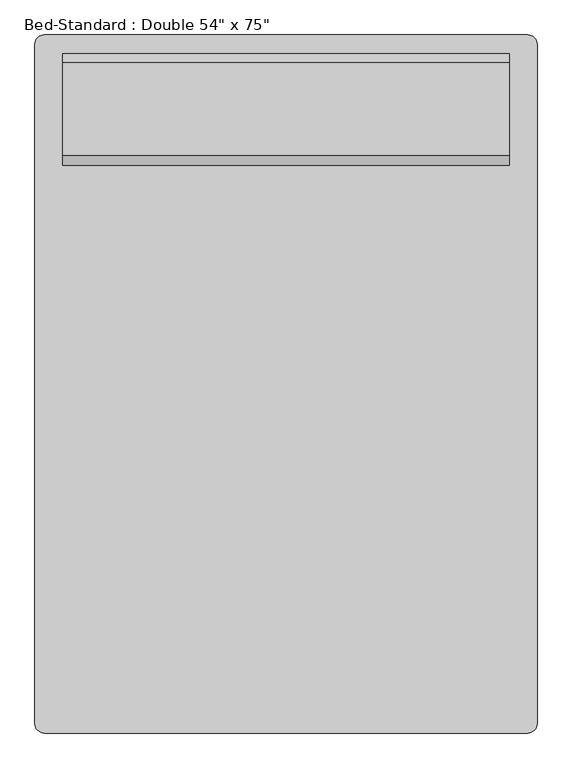
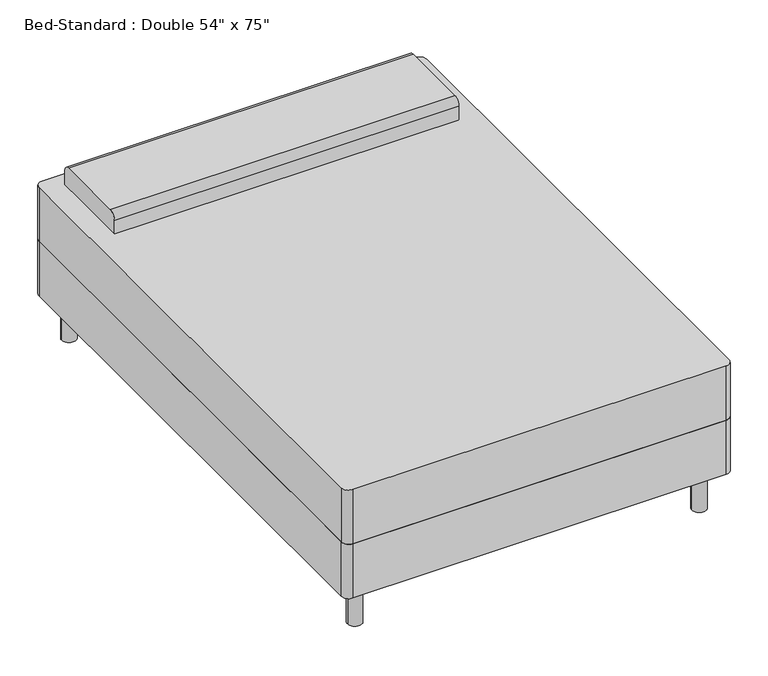
"""IFC4 building model written with IfcOpenShell, lengths in millimetres: furniture geometry."""

from ifc_helpers import new_model, si_unit, point, frame, frame_2d, origin, origin_with_axes, place, context, project, spatial, polyline, circle_curve, trimmed, segment, composite_curve, outline, extrude, source, transform, mapped, element, save


def furniture_0253826f(model_context):
    return source(origin(), model_context, "Body", "SweptSolid", [
        extrude(outline(composite_curve([segment(polyline([(-414.3114754, -972.695082), (-414.3114754, 881.504918)]), True, "CONTINUOUS"), segment(trimmed(circle_curve(frame_2d((-388.9114754, 881.504918)), 25.4), [point((-414.3114754, 881.504918))], [point((-388.9114754, 906.904918))], False, "CARTESIAN"), True, "CONTINUOUS"), segment(polyline([(-388.9114754, 906.904918), (931.8885246, 906.904918)]), True, "CONTINUOUS"), segment(trimmed(circle_curve(frame_2d((931.8885246, 881.504918)), 25.4), [point((931.8885246, 906.904918))], [point((957.2885246, 881.504918))], False, "CARTESIAN"), True, "CONTINUOUS"), segment(polyline([(957.2885246, 881.504918), (957.2885246, -972.695082)]), True, "CONTINUOUS"), segment(trimmed(circle_curve(frame_2d((931.8885246, -972.695082)), 25.4), [point((957.2885246, -972.695082))], [point((931.8885246, -998.095082))], False, "CARTESIAN"), True, "CONTINUOUS"), segment(polyline([(931.8885246, -998.095082), (-388.9114754, -998.095082)]), True, "CONTINUOUS"), segment(trimmed(circle_curve(frame_2d((-388.9114754, -972.695082)), 25.4), [point((-388.9114754, -998.095082))], [point((-414.3114754, -972.695082))], False, "CARTESIAN"), True, "CONTINUOUS")], self_intersect=False)), frame((0.0, 0.0, 152.4), z_axis=(0.0, 0.0, 1.0), x_axis=(1.0, 0.0, 0.0)), (0.0, 0.0, 1.0), 203.2),
        extrude(outline(composite_curve([segment(polyline([(551.304918, 558.8), (551.304918, 609.6)]), True, "CONTINUOUS"), segment(trimmed(circle_curve(frame_2d((576.704918, 609.6)), 25.4), [point((551.304918, 609.6))], [point((576.704918, 635.0))], False, "CARTESIAN"), True, "CONTINUOUS"), segment(polyline([(576.704918, 635.0), (830.704918, 635.0)]), True, "CONTINUOUS"), segment(trimmed(circle_curve(frame_2d((830.704918, 609.6)), 25.4), [point((830.704918, 635.0))], [point((856.104918, 609.6))], False, "CARTESIAN"), True, "CONTINUOUS"), segment(polyline([(856.104918, 609.6), (856.104918, 558.8), (551.304918, 558.8)]), True, "CONTINUOUS")], self_intersect=False)), frame((-338.1114754, 0.0, 0.0), z_axis=(1.0, 0.0, 0.0), x_axis=(0.0, 1.0, 0.0)), (0.0, 0.0, 1.0), 1219.2),
        extrude(outline(composite_curve([segment(trimmed(circle_curve(frame_2d((-338.1114754, 830.704918)), 25.4), [point((-363.5114754, 830.704918))], [point((-312.7114754, 830.704918))], False, "CARTESIAN"), True, "CONTINUOUS"), segment(trimmed(circle_curve(frame_2d((-338.1114754, 830.704918)), 25.4), [point((-312.7114754, 830.704918))], [point((-363.5114754, 830.704918))], False, "CARTESIAN"), True, "CONTINUOUS")], self_intersect=False)), origin_with_axes(), (0.0, 0.0, 1.0), 152.4),
        extrude(outline(composite_curve([segment(trimmed(circle_curve(frame_2d((881.0885246, 830.704918)), 25.4), [point((855.6885246, 830.704918))], [point((906.4885246, 830.704918))], False, "CARTESIAN"), True, "CONTINUOUS"), segment(trimmed(circle_curve(frame_2d((881.0885246, 830.704918)), 25.4), [point((906.4885246, 830.704918))], [point((855.6885246, 830.704918))], False, "CARTESIAN"), True, "CONTINUOUS")], self_intersect=False)), origin_with_axes(), (0.0, 0.0, 1.0), 152.4),
        extrude(outline(composite_curve([segment(trimmed(circle_curve(frame_2d((881.0885246, -921.895082)), 25.4), [point((855.6885246, -921.895082))], [point((906.4885246, -921.895082))], False, "CARTESIAN"), True, "CONTINUOUS"), segment(trimmed(circle_curve(frame_2d((881.0885246, -921.895082)), 25.4), [point((906.4885246, -921.895082))], [point((855.6885246, -921.895082))], False, "CARTESIAN"), True, "CONTINUOUS")], self_intersect=False)), origin_with_axes(), (0.0, 0.0, 1.0), 152.4),
        extrude(outline(composite_curve([segment(trimmed(circle_curve(frame_2d((-338.1114754, -921.895082)), 25.4), [point((-363.5114754, -921.895082))], [point((-312.7114754, -921.895082))], False, "CARTESIAN"), True, "CONTINUOUS"), segment(trimmed(circle_curve(frame_2d((-338.1114754, -921.895082)), 25.4), [point((-312.7114754, -921.895082))], [point((-363.5114754, -921.895082))], False, "CARTESIAN"), True, "CONTINUOUS")], self_intersect=False)), origin_with_axes(), (0.0, 0.0, 1.0), 152.4),
        extrude(outline(composite_curve([segment(polyline([(-388.9114754, 906.904918), (931.8885246, 906.904918)]), True, "CONTINUOUS"), segment(trimmed(circle_curve(frame_2d((931.8885246, 881.504918)), 25.4), [point((931.8885246, 906.904918))], [point((957.2885246, 881.504918))], False, "CARTESIAN"), True, "CONTINUOUS"), segment(polyline([(957.2885246, 881.504918), (957.2885246, -972.695082)]), True, "CONTINUOUS"), segment(trimmed(circle_curve(frame_2d((931.8885246, -972.695082)), 25.4), [point((957.2885246, -972.695082))], [point((931.8885246, -998.095082))], False, "CARTESIAN"), True, "CONTINUOUS"), segment(polyline([(931.8885246, -998.095082), (-388.9114754, -998.095082)]), True, "CONTINUOUS"), segment(trimmed(circle_curve(frame_2d((-388.9114754, -972.695082)), 25.4), [point((-388.9114754, -998.095082))], [point((-414.3114754, -972.695082))], False, "CARTESIAN"), True, "CONTINUOUS"), segment(polyline([(-414.3114754, -972.695082), (-414.3114754, 881.504918)]), True, "CONTINUOUS"), segment(trimmed(circle_curve(frame_2d((-388.9114754, 881.504918)), 25.4), [point((-414.3114754, 881.504918))], [point((-388.9114754, 906.904918))], False, "CARTESIAN"), True, "CONTINUOUS")], self_intersect=False)), frame((0.0, 0.0, 355.6), z_axis=(0.0, 0.0, 1.0), x_axis=(1.0, 0.0, 0.0)), (0.0, 0.0, 1.0), 203.2),
    ])


if __name__ == "__main__":
    model = new_model("IFC4")
    model_context = context("Model", 3, world=origin())
    ifc_project = project(units=[si_unit("LENGTHUNIT", "METRE", prefix="MILLI")], contexts=[model_context])
    site = spatial("IfcSite", under=ifc_project)
    building = spatial("IfcBuilding", under=site)
    placement = place(None, origin())
    furniture_shape = furniture_0253826f(model_context)
    element("IfcFurniture", 1, ObjectType="Bed-Standard : Double 54\" x 75\"", at=placement, inside=building, context=model_context, shape_type="MappedRepresentation", body=[
        mapped(furniture_shape, transform((0.0, 0.0, 0.0), x_axis=(1.0, 0.0, 0.0), y_axis=(0.0, 1.0, 0.0), z_axis=(0.0, 0.0, 1.0))),
    ])
    save(model, "model.ifc")

# Revit data of these elements
# Type "Bed-Standard : Double 54\" x 75\""
#   Assembly Code = "E2020200"
#   Length = 6' - 3"
#   Width = 4' - 6"
#   Leg Material = Steel, Chrome Plated
#   Mattress Material = Linen, White
#   Default Elevation = 0
# Element 1 (IfcFurniture, "Bed-Standard : Double 54\" x 75\"")
#   Materials on its faces: "Linen, White", "Steel, Chrome Plated"
# Materials
#   "Steel, Chrome Plated": class "Metal", colour RGB 17 17 17, transparency 0, Description = "Chromiuim plated steel", Cost = 0
#   "Linen, White": class "Textile", colour RGB 247 247 239, transparency 0, Description = "Linen, white", Cost = 0
